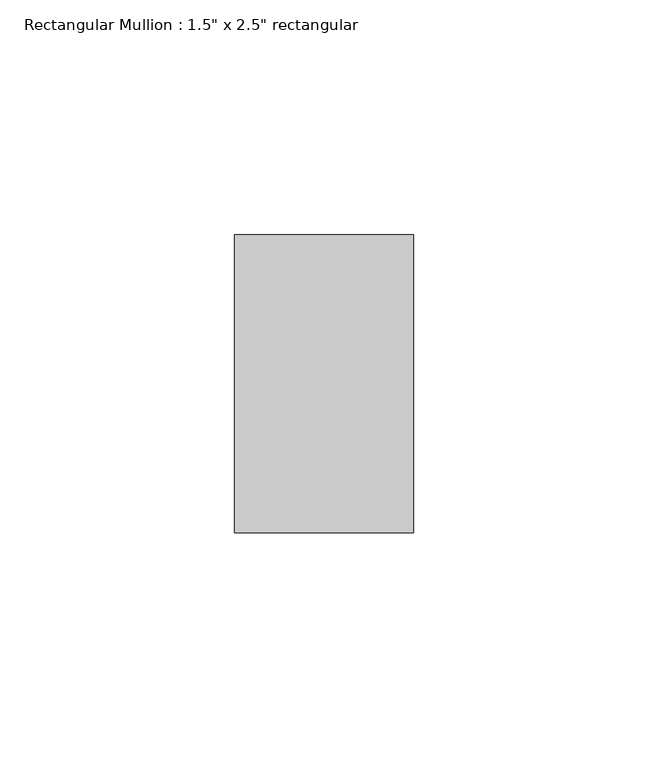
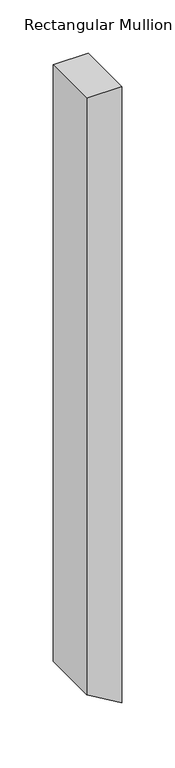
"""IFC4 building model written with IfcOpenShell, lengths in millimetres: member geometry."""

from ifc_helpers import new_model, si_unit, frame, origin, place, context, project, spatial, polyline, outline, extrude, source, transform, mapped, element, save


def member_1ba99afd(model_context):
    return source(origin(), model_context, "Body", "SweptSolid", [
        extrude(outline(polyline([(0.0, 0.0), (0.0, -38.1), (-686.4974369, -38.1), (-709.1419508, 0.0), (0.0, 0.0)])), frame((0.0, -31.75, 0.0), z_axis=(0.0, 1.0, 0.0), x_axis=(0.0, 0.0, 1.0)), (0.0, 0.0, 1.0), 63.5),
    ])


if __name__ == "__main__":
    model = new_model("IFC4")
    model_context = context("Model", 3, world=origin())
    ifc_project = project(units=[si_unit("LENGTHUNIT", "METRE", prefix="MILLI")], contexts=[model_context])
    site = spatial("IfcSite", under=ifc_project)
    building = spatial("IfcBuilding", under=site)
    placement = place(None, origin())
    member_shape = member_1ba99afd(model_context)
    element("IfcMember", 1, ObjectType="Rectangular Mullion : 1.5\" x 2.5\" rectangular", at=placement, inside=building, context=model_context, shape_type="MappedRepresentation", body=[
        mapped(member_shape, transform((0.0, 0.0, 0.0), x_axis=(1.0, 0.0, 0.0), y_axis=(0.0, 1.0, 0.0), z_axis=(0.0, 0.0, 1.0))),
    ])
    save(model, "model.ifc")

# Revit data of these elements
# Type "Rectangular Mullion : 1.5\" x 2.5\" rectangular"
#   built-in parameter 1007304 = 0.208333 (stored number, unit not read)
#   built-in parameter 1007301 = 0.0625 (stored number, unit not read)
#   built-in parameter 1007300 = 0.0625 (stored number, unit not read)
